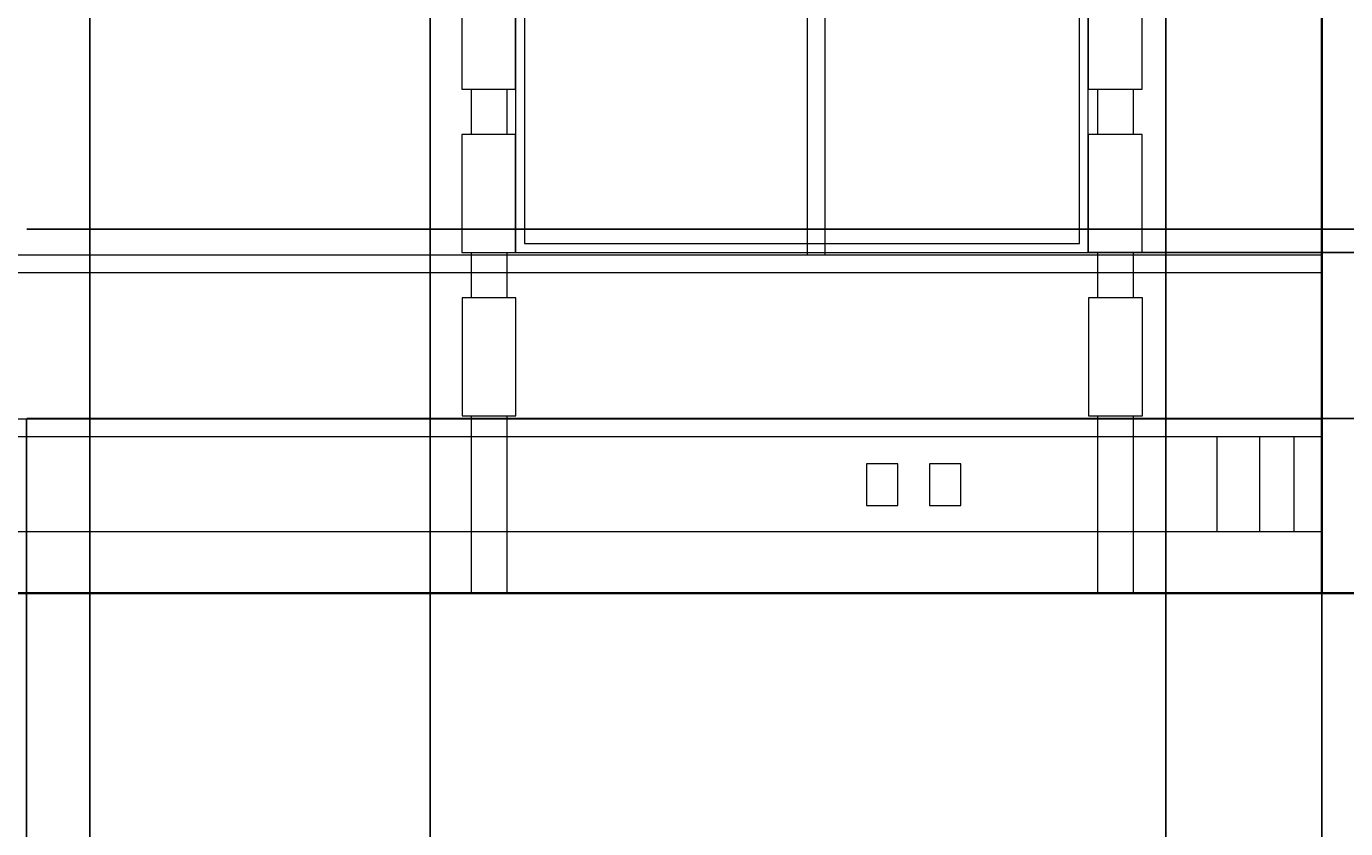
# Model space of a CAD drawing. Units: inches. Extents: x 69 to 650, y -16 to 573.
# Tile 19 of 26: x 383 to 531, y 218 to 308. Entities that reach past the tile are written whole.
import ezdxf

# ---------------------------------------------------------------- set-up
doc = ezdxf.new("R2010")
doc.units = ezdxf.units.IN
doc.header["$MEASUREMENT"] = 0
for name, color, linetype, lineweight in [('A-ANNO-DIMS', 2, 'Continuous', 18), ('A-ELEV', 8, 'Continuous', 18), ('A-GLAZ', 4, 'Continuous', 18), ('A-WALL', 7, 'Continuous', 35)]:
    doc.layers.add(name, color=color, linetype=linetype, lineweight=lineweight)
doc.styles.get("Standard").update_dxf_attribs({"font": 'arial.ttf'})
doc.dimstyles.get("Standard").update_dxf_attribs({"dimtxt": 0.8125, "dimasz": 0.18, "dimexe": 0.18, "dimexo": 0.0625, "dimgap": 0.09, "dimtad": 0, "dimtih": 1, "dimtoh": 1, "dimdec": 4, "dimzin": 0, "dimdsep": 46, "dimlunit": 4, "dimtxsty": 'Standard', "dimcen": 0.09, "dimadec": 0, "dimazin": 0, "dimtfac": 1, "dimtdec": 4, "dimtofl": 0, "dimtmove": 0, "dimatfit": 3, "dimfxl": 1, "dimtolj": 1, "dimtzin": 0, "dimarcsym": 0})

# ---------------------------------------------------------------- blocks, each defined once
blk = doc.blocks.new('WIN-ARCH-SURROUND')
for p, q in [((0, 129.06), (0, 124.83)), ((82.63, 129.06), (0, 129.06)), ((82.63, 124.83), (82.63, 129.06)), ((0, 124.83), (82.63, 124.83)), ((2.69, 109.21), (2.69, 124.83)), ((79.05, 109.21), (79.05, 124.83)), ((3.69, 109.21), (2.69, 109.21)), ((3.69, 109.21), (3.69, 105.89)), ((3.69, 109.21), (78.05, 109.21)), ((7.69, 109.21), (7.69, 105.89)), ((8.73, 105.89), (8.73, 109.21)), ((38.31, 109.21), (38.31, 38)), ((40.31, 109.21), (40.31, 38)), ((74.05, 109.21), (74.05, 105.89)), ((78.05, 109.21), (79.05, 109.21)), ((78.05, 109.21), (78.05, 105.89)), ((3.69, 92.64), (3.69, 87.15)), ((7.69, 92.64), (7.69, 87.15)), ((74.05, 92.64), (74.05, 87.15)), ((78.05, 92.64), (78.05, 87.15)), ((3.69, 73.9), (3.69, 69.84)), ((7.69, 73.9), (7.69, 69.84)), ((74.05, 73.9), (74.05, 69.84)), ((78.05, 73.9), (78.05, 69.84)), ((3.69, 56.59), (3.69, 51.51)), ((7.69, 56.59), (7.69, 51.51)), ((74.05, 56.59), (74.05, 51.51)), ((78.05, 56.59), (78.05, 51.51)), ((3.69, 38.26), (3.69, 33.16)), ((7.69, 38.26), (7.69, 33.16)), ((74.05, 38.26), (74.05, 33.16)), ((78.05, 38.26), (78.05, 33.16)), ((3.69, 19.91), (3.69, 0)), ((7.69, 19.91), (7.69, 0)), ((74.05, 19.91), (74.05, 0)), ((78.05, 19.91), (78.05, 0))]:
    blk.add_line(p, q)
for points in [[(8.73, 109.21), (73.05, 109.21), (73.05, 38.26), (8.73, 38.26)], [(9.73, 108.21), (72.05, 108.21), (72.05, 39.26), (9.73, 39.26)], [(2.69, 105.89), (8.73, 105.89), (8.73, 92.64), (2.69, 92.64)], [(73.05, 105.89), (79.1, 105.89), (79.1, 92.64), (73.05, 92.64)], [(2.69, 87.15), (8.73, 87.15), (8.73, 73.9), (2.69, 73.9)], [(73.05, 87.15), (79.1, 87.15), (79.1, 73.9), (73.05, 73.9)], [(2.69, 69.84), (8.73, 69.84), (8.73, 56.59), (2.69, 56.59)], [(73.05, 69.84), (79.1, 69.84), (79.1, 56.59), (73.05, 56.59)], [(2.69, 51.51), (8.73, 51.51), (8.73, 38.26), (2.69, 38.26)], [(73.05, 51.51), (79.1, 51.51), (79.1, 38.26), (73.05, 38.26)], [(2.65, 33.16), (8.69, 33.16), (8.69, 19.91), (2.65, 19.91)], [(73.01, 33.16), (79.06, 33.16), (79.06, 19.91), (73.01, 19.91)]]:
    blk.add_lwpolyline(points, close=True)
blk.add_ellipse((40.89, 109.21), major_axis=(32.16, 0), ratio=0.165597, start_param=6.283185, end_param=9.424778)
blk = doc.blocks.new('TRIM-FRIEZE-INSET')
blk.add_lwpolyline([(0, 4.66), (3.54, 4.66), (3.54, 0), (0, 0)], close=True)
blk = doc.blocks.new('*D19')
at = {"layer": 'A-ANNO-DIMS', "color": 0, "lineweight": -2, "transparency": 16777216}
for p, q in [((99.56, 471.72), (99.56, 572.74)), ((99.74, 572.56), (358.57, 572.56)), ((619.38, 572.56), (360.54, 572.56)), ((619.56, 87.99), (619.56, 572.74))]:
    blk.add_line(p, q, dxfattribs=at)
at = {"layer": 'A-ANNO-DIMS', "color": 0, "transparency": 16777216}
for points in [[(99.74, 572.59), (99.74, 572.53), (99.56, 572.56)], [(619.38, 572.59), (619.38, 572.53), (619.56, 572.56)]]:
    blk.add_solid(points, dxfattribs=at)
at = {"layer": 'Defpoints', "color": 0, "transparency": 16777216}
for p in [(619.56, 572.56), (99.56, 471.66), (619.56, 87.93)]:
    blk.add_point(p, dxfattribs=at)
at = {"layer": 'A-ANNO-DIMS', "color": 0, "transparency": 16777216, "insert": (359.56, 572.56), "char_height": 0.812, "attachment_point": 5}
blk.add_mtext('\\A1;520', dxfattribs=at)
blk = doc.blocks.new('*D20')
at = {"layer": 'A-ANNO-DIMS', "color": 0, "lineweight": -2, "transparency": 16777216}
for p, q in [((504.24, 544.16), (648.14, 544.16)), ((647.96, 543.98), (647.96, 304.55)), ((647.96, 64.11), (647.96, 303.54)), ((619.62, 63.93), (648.14, 63.93))]:
    blk.add_line(p, q, dxfattribs=at)
at = {"layer": 'A-ANNO-DIMS', "color": 0, "transparency": 16777216}
for points in [[(647.93, 543.98), (647.99, 543.98), (647.96, 544.16)], [(647.93, 64.11), (647.99, 64.11), (647.96, 63.93)]]:
    blk.add_solid(points, dxfattribs=at)
at = {"layer": 'Defpoints', "color": 0, "transparency": 16777216}
for p in [(504.18, 544.16), (647.96, 544.16), (619.56, 63.93)]:
    blk.add_point(p, dxfattribs=at)
at = {"layer": 'A-ANNO-DIMS', "color": 0, "transparency": 16777216, "insert": (647.96, 304.04), "char_height": 0.812, "attachment_point": 5}
blk.add_mtext('\\A1;480.2', dxfattribs=at)
blk = doc.blocks.new('*D25')
at = {"layer": 'A-ANNO-DIMS', "color": 0, "lineweight": -2, "transparency": 16777216}
for p, q in [((99.49, 243.93), (70.98, 243.93)), ((71.16, 243.75), (71.16, 228.3)), ((71.16, 211.83), (71.16, 227.29)), ((441.88, 211.65), (70.98, 211.65))]:
    blk.add_line(p, q, dxfattribs=at)
at = {"layer": 'A-ANNO-DIMS', "color": 0, "transparency": 16777216}
for points in [[(71.13, 243.75), (71.19, 243.75), (71.16, 243.93)], [(71.13, 211.83), (71.19, 211.83), (71.16, 211.65)]]:
    blk.add_solid(points, dxfattribs=at)
at = {"layer": 'Defpoints', "color": 0, "transparency": 16777216}
for p in [(71.16, 243.93), (99.56, 243.93), (441.94, 211.65)]:
    blk.add_point(p, dxfattribs=at)
at = {"layer": 'A-ANNO-DIMS', "color": 0, "transparency": 16777216, "insert": (71.16, 227.79), "char_height": 0.812, "attachment_point": 5}
blk.add_mtext('\\A1;32.28', dxfattribs=at)
blk = doc.blocks.new('*D38')
at = {"layer": 'A-ANNO-DIMS', "color": 0, "lineweight": -2, "transparency": 16777216}
for p, q in [((307.8, 384.84), (307.8, 35.35)), ((390.43, 384.84), (390.43, 35.35)), ((307.98, 35.53), (347.65, 35.53)), ((390.25, 35.53), (350.57, 35.53))]:
    blk.add_line(p, q, dxfattribs=at)
at = {"layer": 'A-ANNO-DIMS', "color": 0, "transparency": 16777216}
for points in [[(307.98, 35.56), (307.98, 35.5), (307.8, 35.53)], [(390.25, 35.56), (390.25, 35.5), (390.43, 35.53)]]:
    blk.add_solid(points, dxfattribs=at)
at = {"layer": 'Defpoints', "color": 0, "transparency": 16777216}
for p in [(307.8, 384.9), (390.43, 384.9), (390.43, 35.53)]:
    blk.add_point(p, dxfattribs=at)
at = {"layer": 'A-ANNO-DIMS', "color": 0, "transparency": 16777216, "insert": (349.11, 35.53), "char_height": 0.812, "attachment_point": 5}
blk.add_mtext('\\A1;82.63', dxfattribs=at)
blk = doc.blocks.new('*D39')
at = {"layer": 'A-ANNO-DIMS', "color": 0, "lineweight": -2, "transparency": 16777216}
for p, q in [((390.43, 384.84), (390.43, 35.35)), ((428.66, 372.93), (428.66, 35.35)), ((390.61, 35.53), (407.77, 35.53)), ((428.48, 35.53), (411.32, 35.53))]:
    blk.add_line(p, q, dxfattribs=at)
at = {"layer": 'A-ANNO-DIMS', "color": 0, "transparency": 16777216}
for points in [[(390.61, 35.56), (390.61, 35.5), (390.43, 35.53)], [(428.48, 35.56), (428.48, 35.5), (428.66, 35.53)]]:
    blk.add_solid(points, dxfattribs=at)
at = {"layer": 'Defpoints', "color": 0, "transparency": 16777216}
for p in [(390.43, 384.9), (428.66, 372.99), (428.66, 35.53)]:
    blk.add_point(p, dxfattribs=at)
at = {"layer": 'A-ANNO-DIMS', "color": 0, "transparency": 16777216, "insert": (409.55, 35.53), "char_height": 0.812, "attachment_point": 5}
blk.add_mtext('\\A1;38.236', dxfattribs=at)
blk = doc.blocks.new('*D40')
at = {"layer": 'A-ANNO-DIMS', "color": 0, "lineweight": -2, "transparency": 16777216}
for p, q in [((511.3, 372.93), (511.3, 35.35)), ((528.81, 243.87), (528.81, 35.35)), ((511.48, 35.53), (518.32, 35.53)), ((528.63, 35.53), (521.79, 35.53))]:
    blk.add_line(p, q, dxfattribs=at)
at = {"layer": 'A-ANNO-DIMS', "color": 0, "transparency": 16777216}
for points in [[(511.48, 35.56), (511.48, 35.5), (511.3, 35.53)], [(528.63, 35.56), (528.63, 35.5), (528.81, 35.53)]]:
    blk.add_solid(points, dxfattribs=at)
at = {"layer": 'Defpoints', "color": 0, "transparency": 16777216}
for p in [(511.3, 372.99), (528.81, 243.93), (528.81, 35.53)]:
    blk.add_point(p, dxfattribs=at)
at = {"layer": 'A-ANNO-DIMS', "color": 0, "transparency": 16777216, "insert": (520.06, 35.53), "char_height": 0.812, "attachment_point": 5}
blk.add_mtext('\\A1;17.514', dxfattribs=at)
blk = doc.blocks.new('*D41')
at = {"layer": 'A-ANNO-DIMS', "color": 0, "lineweight": -2, "transparency": 16777216}
for p, q in [((528.81, 243.87), (528.81, 35.35)), ((619.56, 243.87), (619.56, 35.35)), ((528.99, 35.53), (572.72, 35.53)), ((619.38, 35.53), (575.64, 35.53))]:
    blk.add_line(p, q, dxfattribs=at)
at = {"layer": 'A-ANNO-DIMS', "color": 0, "transparency": 16777216}
for points in [[(528.99, 35.56), (528.99, 35.5), (528.81, 35.53)], [(619.38, 35.56), (619.38, 35.5), (619.56, 35.53)]]:
    blk.add_solid(points, dxfattribs=at)
at = {"layer": 'Defpoints', "color": 0, "transparency": 16777216}
for p in [(528.81, 243.93), (619.56, 243.93), (619.56, 35.53)]:
    blk.add_point(p, dxfattribs=at)
at = {"layer": 'A-ANNO-DIMS', "color": 0, "transparency": 16777216, "insert": (574.18, 35.53), "char_height": 0.812, "attachment_point": 5}
blk.add_mtext('\\A1;90.74', dxfattribs=at)
blk = doc.blocks.new('*D42')
at = {"layer": 'A-ANNO-DIMS', "color": 0, "lineweight": -2, "transparency": 16777216}
for p, q in [((502.63, 282.19), (648.14, 282.19)), ((647.96, 282.01), (647.96, 263.57)), ((647.96, 244.11), (647.96, 262.56)), ((507.67, 243.93), (648.14, 243.93))]:
    blk.add_line(p, q, dxfattribs=at)
at = {"layer": 'A-ANNO-DIMS', "color": 0, "transparency": 16777216}
for points in [[(647.93, 282.01), (647.99, 282.01), (647.96, 282.19)], [(647.93, 244.11), (647.99, 244.11), (647.96, 243.93)]]:
    blk.add_solid(points, dxfattribs=at)
at = {"layer": 'Defpoints', "color": 0, "transparency": 16777216}
for p in [(502.56, 282.19), (647.96, 282.19), (507.61, 243.93)]:
    blk.add_point(p, dxfattribs=at)
at = {"layer": 'A-ANNO-DIMS', "color": 0, "transparency": 16777216, "insert": (647.96, 263.06), "char_height": 0.812, "attachment_point": 5}
blk.add_mtext('\\A1;38.26', dxfattribs=at)
blk = doc.blocks.new('*D43')
at = {"layer": 'A-ANNO-DIMS', "color": 0, "lineweight": -2, "transparency": 16777216}
for p, q in [((502.63, 353.14), (648.14, 353.14)), ((647.96, 352.96), (647.96, 318.17)), ((647.96, 282.37), (647.96, 317.16)), ((502.63, 282.19), (648.14, 282.19))]:
    blk.add_line(p, q, dxfattribs=at)
at = {"layer": 'A-ANNO-DIMS', "color": 0, "transparency": 16777216}
for points in [[(647.93, 352.96), (647.99, 352.96), (647.96, 353.14)], [(647.93, 282.37), (647.99, 282.37), (647.96, 282.19)]]:
    blk.add_solid(points, dxfattribs=at)
at = {"layer": 'Defpoints', "color": 0, "transparency": 16777216}
for p in [(502.56, 353.14), (647.96, 353.14), (502.56, 282.19)]:
    blk.add_point(p, dxfattribs=at)
at = {"layer": 'A-ANNO-DIMS', "color": 0, "transparency": 16777216, "insert": (647.96, 317.67), "char_height": 0.812, "attachment_point": 5}
blk.add_mtext('\\A1;70.95', dxfattribs=at)
blk = doc.blocks.new('*D71')
at = {"layer": 'A-ANNO-DIMS', "color": 0, "lineweight": -2, "transparency": 16777216}
for p, q in [((370.73, 263.46), (370.73, 35.35)), ((383.3, 263.46), (383.3, 35.35)), ((370.91, 35.53), (375.59, 35.53)), ((383.12, 35.53), (378.44, 35.53))]:
    blk.add_line(p, q, dxfattribs=at)
at = {"layer": 'A-ANNO-DIMS', "color": 0, "transparency": 16777216}
for points in [[(370.91, 35.56), (370.91, 35.5), (370.73, 35.53)], [(383.12, 35.56), (383.12, 35.5), (383.3, 35.53)]]:
    blk.add_solid(points, dxfattribs=at)
at = {"layer": 'Defpoints', "color": 0, "transparency": 16777216}
for p in [(370.73, 263.53), (383.3, 263.53), (383.3, 35.53)]:
    blk.add_point(p, dxfattribs=at)
at = {"layer": 'A-ANNO-DIMS', "color": 0, "transparency": 16777216, "insert": (377.02, 35.53), "char_height": 0.812, "attachment_point": 5}
blk.add_mtext('\\A1;12.57', dxfattribs=at)
blk = doc.blocks.new('*D72')
at = {"layer": 'A-ANNO-DIMS', "color": 0, "lineweight": -2, "transparency": 16777216}
for p, q in [((383.36, 284.81), (648.14, 284.81)), ((647.96, 284.63), (647.96, 274.67)), ((647.96, 263.71), (647.96, 273.66)), ((383.36, 263.53), (648.14, 263.53))]:
    blk.add_line(p, q, dxfattribs=at)
at = {"layer": 'A-ANNO-DIMS', "color": 0, "transparency": 16777216}
for points in [[(647.93, 284.63), (647.99, 284.63), (647.96, 284.81)], [(647.93, 263.71), (647.99, 263.71), (647.96, 263.53)]]:
    blk.add_solid(points, dxfattribs=at)
at = {"layer": 'Defpoints', "color": 0, "transparency": 16777216}
for p in [(383.3, 284.81), (647.96, 284.81), (383.3, 263.53)]:
    blk.add_point(p, dxfattribs=at)
at = {"layer": 'A-ANNO-DIMS', "color": 0, "transparency": 16777216, "insert": (647.96, 274.17), "char_height": 0.812, "attachment_point": 5}
blk.add_mtext('\\A1;21.287', dxfattribs=at)
blk = doc.blocks.new('*D73')
at = {"layer": 'A-ANNO-DIMS', "color": 0, "lineweight": -2, "transparency": 16777216}
for p, q in [((383.36, 319.57), (648.14, 319.57)), ((647.96, 319.39), (647.96, 302.7)), ((647.96, 284.99), (647.96, 301.69)), ((383.36, 284.81), (648.14, 284.81))]:
    blk.add_line(p, q, dxfattribs=at)
at = {"layer": 'A-ANNO-DIMS', "color": 0, "transparency": 16777216}
for points in [[(647.93, 319.39), (647.99, 319.39), (647.96, 319.57)], [(647.93, 284.99), (647.99, 284.99), (647.96, 284.81)]]:
    blk.add_solid(points, dxfattribs=at)
at = {"layer": 'Defpoints', "color": 0, "transparency": 16777216}
for p in [(383.3, 319.57), (647.96, 319.57), (383.3, 284.81)]:
    blk.add_point(p, dxfattribs=at)
at = {"layer": 'A-ANNO-DIMS', "color": 0, "transparency": 16777216, "insert": (647.96, 302.19), "char_height": 0.812, "attachment_point": 5}
blk.add_mtext('\\A1;34.76', dxfattribs=at)

msp = doc.modelspace()

# ---------------------------------------------------------------- linework, layer by layer
at = {"layer": 'A-ELEV'}
for p, q in [((190.299, 281.93), (528.812, 281.93)), ((190.299, 279.93), (528.812, 279.93)), ((190.299, 263.5253), (528.812, 263.5253)), ((190.299, 261.5253), (528.812, 261.5253)), ((517.0259, 261.5253), (517.0259, 250.8759)), ((521.8168, 261.5253), (521.8168, 250.8759)), ((525.6408, 261.5253), (525.6408, 250.8759)), ((190.299, 250.8759), (484.5159, 250.8759)), ((484.5159, 250.8759), (528.812, 250.8759))]:
    msp.add_line(p, q, dxfattribs=at)
at = {"layer": 'A-WALL'}
msp.add_line((99.556, 243.93), (619.555, 243.93), dxfattribs=at)
msp.add_lwpolyline([(619.555, 363.8739), (528.812, 363.8739), (528.812, 243.93), (619.555, 243.93)], close=True, dxfattribs=at)

# ---------------------------------------------------------------- block references
at = {"layer": 'A-ELEV', "extrusion": (0, 0, -1), "zscale": -1}
for p in [(-481.1939, 253.792), (-488.267, 253.792)]:
    msp.add_blockref('TRIM-FRIEZE-INSET', p, dxfattribs=at)
at = {"layer": 'A-GLAZ', "extrusion": (0, 0, -1), "zscale": -1}
msp.add_blockref('WIN-ARCH-SURROUND', (-511.298, 243.93), dxfattribs=at)

# ---------------------------------------------------------------- dimensions: what is measured, and where the dimension line sits
at = {"layer": 'A-ANNO-DIMS'}
for base, p1, p2, override, picture, middle in [((619.555, 572.5573), (99.556, 471.6595), (619.555, 87.93), {"dimdec": 0, "dimlfac": 1, "dimrnd": 0, "dimzin": 0, "dimdsep": 46, "dimlunit": 2}, '*D19', (359.5555, 572.5573)), ((390.4291, 35.53), (307.7955, 384.8986), (390.4291, 384.8986), {"dimdec": 2, "dimlfac": 1, "dimrnd": 0, "dimzin": 0, "dimdsep": 46, "dimlunit": 2}, '*D38', (349.1123, 35.53)), ((428.6648, 35.53), (390.4291, 384.8986), (428.6648, 372.9907), {"dimdec": 3, "dimlfac": 1, "dimrnd": 0, "dimzin": 0, "dimdsep": 46, "dimlunit": 2}, '*D39', (409.547, 35.53)), ((528.812, 35.53), (511.2984, 372.9907), (528.812, 243.93), {"dimdec": 3, "dimlfac": 1, "dimrnd": 0, "dimzin": 0, "dimdsep": 46, "dimlunit": 2}, '*D40', (520.0552, 35.53)), ((383.3022, 35.53), (370.7319, 263.5253), (383.3022, 263.5253), {"dimdec": 2, "dimlfac": 1, "dimrnd": 0, "dimzin": 0, "dimdsep": 46, "dimlunit": 2}, '*D71', (377.0171, 35.53)), ((619.555, 35.53), (528.812, 243.93), (619.555, 243.93), {"dimdec": 2, "dimlfac": 1, "dimrnd": 0, "dimzin": 0, "dimdsep": 46, "dimlunit": 2}, '*D41', (574.1835, 35.53))]:
    dim = msp.add_linear_dim(base=base, p1=p1, p2=p2, dimstyle='Standard', override=override, dxfattribs=at)
    dim.commit()
    dim.dimension.update_dxf_attribs({"geometry": picture, "text_midpoint": middle})
for base, p1, p2, override, picture, middle in [((647.955, 544.1573), (619.555, 63.93), (504.1763, 544.1573), {"dimdec": 1, "dimlfac": 1, "dimrnd": 0, "dimzin": 0, "dimdsep": 46, "dimlunit": 2}, '*D20', (647.955, 304.0436)), ((647.955, 353.1381), (502.5637, 282.1923), (502.5637, 353.1381), {"dimdec": 2, "dimlfac": 1, "dimrnd": 0, "dimzin": 0, "dimdsep": 46, "dimlunit": 2}, '*D43', (647.955, 317.6652)), ((647.955, 319.5737), (383.3022, 284.812), (383.3022, 319.5737), {"dimdec": 2, "dimlfac": 1, "dimrnd": 0, "dimzin": 0, "dimdsep": 46, "dimlunit": 2}, '*D73', (647.955, 302.1928)), ((647.955, 284.812), (383.3022, 263.5253), (383.3022, 284.812), {"dimdec": 3, "dimlfac": 1, "dimrnd": 0, "dimzin": 0, "dimdsep": 46, "dimlunit": 2}, '*D72', (647.955, 274.1686)), ((647.955, 282.1923), (507.611, 243.93), (502.5637, 282.1923), {"dimdec": 2, "dimlfac": 1, "dimrnd": 0, "dimzin": 0, "dimdsep": 46, "dimlunit": 2}, '*D42', (647.955, 263.0612)), ((71.156, 243.93), (441.9398, 211.6519), (99.556, 243.93), {"dimdec": 2, "dimlfac": 1, "dimrnd": 0, "dimzin": 0, "dimdsep": 46, "dimlunit": 2}, '*D25', (71.156, 227.7909))]:
    dim = msp.add_linear_dim(base=base, p1=p1, p2=p2, angle=90, dimstyle='Standard', override=override, dxfattribs=at)
    dim.commit()
    dim.dimension.update_dxf_attribs({"geometry": picture, "text_midpoint": middle})

doc.saveas('drawing.dxf')
